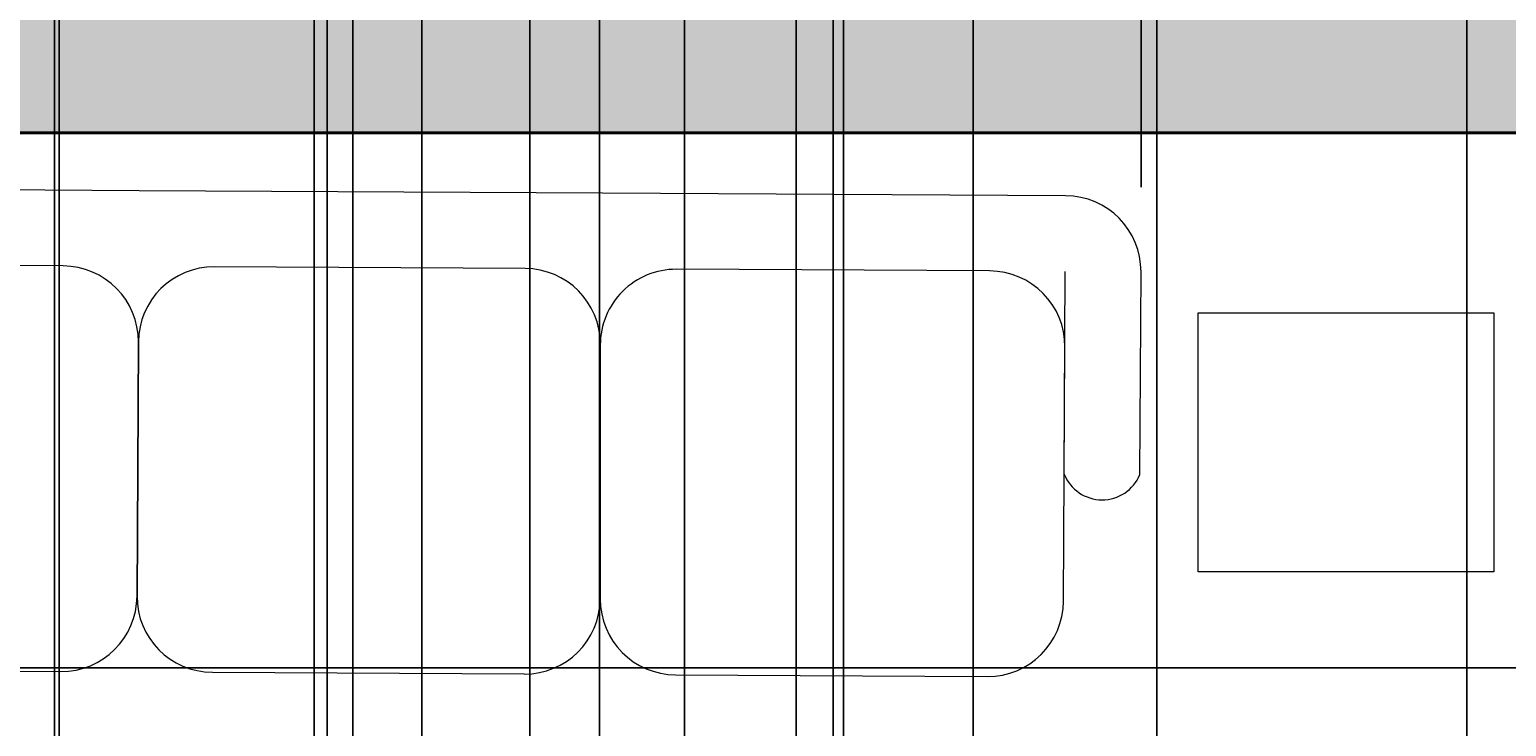
# Model space of a CAD drawing. Units: inches. Extents: x 818 to 1898, y 976 to 2364.
# Tile 31 of 96: x 1282 to 1391, y 1643 to 1695. Entities that reach past the tile are written whole.
import ezdxf

# ---------------------------------------------------------------- set-up
doc = ezdxf.new("R2010")
doc.units = ezdxf.units.IN
doc.header["$LTSCALE"] = 5
doc.header["$MEASUREMENT"] = 0
for name, color, linetype, lineweight in [('A-ANNO-DIMS', 2, 'Continuous', 18), ('A-FURN', 8, 'Continuous', 18), ('A-WALL', 7, 'Continuous', 40)]:
    doc.layers.add(name, color=color, linetype=linetype, lineweight=lineweight)
doc.layers.add('A-WALL-PATT', color=251, linetype='Continuous', lineweight=13, true_color=0x636466)
doc.styles.get("Standard").update_dxf_attribs({"font": 'arial.ttf'})
doc.dimstyles.get("Standard").update_dxf_attribs({"dimtxt": 0.18, "dimasz": 0.18, "dimexe": 0.18, "dimexo": 0.0625, "dimgap": 0.09, "dimtad": 0, "dimtih": 1, "dimtoh": 1, "dimdec": 4, "dimzin": 0, "dimdsep": 46, "dimtxsty": 'Standard', "dimcen": 0.09, "dimadec": 0, "dimazin": 0, "dimtfac": 1, "dimtdec": 4, "dimtofl": 0, "dimtmove": 0, "dimatfit": 3, "dimfxl": 1, "dimtolj": 1, "dimtzin": 0, "dimarcsym": 0})

# ---------------------------------------------------------------- blocks, each defined once
blk = doc.blocks.new('SOFA-3-SEAT')
for p, q in [((39.87, 35.86), (5.7, 36.05)), ((74.05, 35.68), (39.88, 35.86)), ((108.23, 35.49), (74.06, 35.68)), ((34.25, 30.31), (11.25, 30.43)), ((68.34, 30.12), (45.43, 30.24)), ((102.62, 29.94), (79.51, 30.06)), ((108.12, 14.94), (108.2, 29.9)), ((113.71, 14.91), (113.79, 29.87)), ((39.71, 5.93), (39.81, 24.69)), ((39.82, 24.69), (39.72, 5.93)), ((73.9, 5.71), (73.9, 24.47)), ((108.07, 5.56), (108.17, 24.32)), ((11.09, 0.49), (34.09, 0.37)), ((45.27, 0.31), (68.27, 0.19)), ((79.45, 0.12), (102.45, 0))]:
    blk.add_line(p, q)
for centre, radius, start, end in [((108.2, 29.9), 5.59, 359.6898, 89.6898), ((34.22, 24.72), 5.59, 359.6898, 89.6898), ((45.4, 24.66), 5.59, 89.6898, 179.6898), ((68.31, 24.53), 5.59, 0, 89.6898), ((79.48, 24.47), 5.59, 89.6898, 180), ((102.59, 24.35), 5.59, 359.6898, 89.6898), ((110.92, 16.05), 3.01, 201.7034, 337.6762), ((34.12, 5.96), 5.59, 269.6898, 359.6898), ((45.3, 5.9), 5.59, 179.6898, 269.6898), ((68.3, 5.77), 5.59, 269.6898, 359.6898), ((79.48, 5.71), 5.59, 179.6898, 269.6898), ((102.48, 5.59), 5.59, 269.6898, 359.6898)]:
    blk.add_arc(centre, radius, start, end)
blk = doc.blocks.new('SIDE-TABLE')
blk.add_lwpolyline([(0, 19.12), (21.82, 19.12), (21.82, 0), (0, 0)], close=True)
blk = doc.blocks.new('*D42')
at = {"layer": 'A-ANNO-DIMS', "color": 0, "lineweight": -2, "ltscale": 5, "transparency": 16777216}
for p, q in [((1250.19, 1683.07), (1250.19, 1700.26)), ((1250.37, 1700.08), (1306.12, 1700.08)), ((1363.82, 1700.08), (1308.07, 1700.08)), ((1364, 1683.07), (1364, 1700.26))]:
    blk.add_line(p, q, dxfattribs=at)
at = {"layer": 'A-ANNO-DIMS', "color": 0, "ltscale": 5, "transparency": 16777216}
for points in [[(1250.37, 1700.11), (1250.37, 1700.05), (1250.19, 1700.08)], [(1363.82, 1700.11), (1363.82, 1700.05), (1364, 1700.08)]]:
    blk.add_solid(points, dxfattribs=at)
at = {"layer": 'Defpoints', "color": 0, "ltscale": 5, "transparency": 16777216}
for p in [(1364, 1700.08), (1250.19, 1683.01), (1364, 1683.01)]:
    blk.add_point(p, dxfattribs=at)
at = {"layer": 'A-ANNO-DIMS', "color": 0, "ltscale": 5, "transparency": 16777216, "insert": (1307.1, 1700.08), "char_height": 0.18, "attachment_point": 5}
blk.add_mtext('\\A1;SOFA 114 TYP.', dxfattribs=at)
blk = doc.blocks.new('*D61')
at = {"layer": 'A-ANNO-DIMS', "color": 0, "lineweight": -2, "ltscale": 5, "transparency": 16777216}
for p, q in [((1071.73, 1203.03), (1071.73, 2363.87)), ((1071.91, 2363.69), (1250.94, 2363.69)), ((1430.55, 2363.69), (1251.51, 2363.69)), ((1430.73, 1203.03), (1430.73, 2363.87))]:
    blk.add_line(p, q, dxfattribs=at)
at = {"layer": 'A-ANNO-DIMS', "color": 0, "ltscale": 5, "transparency": 16777216}
for points in [[(1071.91, 2363.72), (1071.91, 2363.66), (1071.73, 2363.69)], [(1430.55, 2363.72), (1430.55, 2363.66), (1430.73, 2363.69)]]:
    blk.add_solid(points, dxfattribs=at)
at = {"layer": 'Defpoints', "color": 0, "ltscale": 5, "transparency": 16777216}
for p in [(1430.73, 2363.69), (1071.73, 1202.96), (1430.73, 1202.96)]:
    blk.add_point(p, dxfattribs=at)
at = {"layer": 'A-ANNO-DIMS', "color": 0, "ltscale": 5, "transparency": 16777216, "insert": (1251.23, 2363.69), "char_height": 0.18, "attachment_point": 5}
blk.add_mtext('\\A1;359', dxfattribs=at)
blk = doc.blocks.new('*D64')
at = {"layer": 'A-ANNO-DIMS', "color": 0, "lineweight": -2, "ltscale": 5, "transparency": 16777216}
for p, q in [((1197.73, 1501.14), (1197.73, 2363.87)), ((1197.91, 2363.69), (1313.93, 2363.69)), ((1430.55, 2363.69), (1314.52, 2363.69)), ((1430.73, 1501.14), (1430.73, 2363.87))]:
    blk.add_line(p, q, dxfattribs=at)
at = {"layer": 'A-ANNO-DIMS', "color": 0, "ltscale": 5, "transparency": 16777216}
for points in [[(1197.91, 2363.72), (1197.91, 2363.66), (1197.73, 2363.69)], [(1430.55, 2363.72), (1430.55, 2363.66), (1430.73, 2363.69)]]:
    blk.add_solid(points, dxfattribs=at)
at = {"layer": 'Defpoints', "color": 0, "ltscale": 5, "transparency": 16777216}
for p in [(1430.73, 2363.69), (1197.73, 1501.08), (1430.73, 1501.08)]:
    blk.add_point(p, dxfattribs=at)
at = {"layer": 'A-ANNO-DIMS', "color": 0, "ltscale": 5, "transparency": 16777216, "insert": (1314.23, 2363.69), "char_height": 0.18, "attachment_point": 5}
blk.add_mtext('\\A1;233', dxfattribs=at)
blk = doc.blocks.new('*D96')
at = {"layer": 'A-ANNO-DIMS', "color": 0, "lineweight": -2, "ltscale": 5, "transparency": 16777216}
for p, q in [((1229.65, 1071.12), (1229.65, 2363.87)), ((1229.83, 2363.69), (1256.52, 2363.69)), ((1283.99, 2363.69), (1257.3, 2363.69)), ((1284.17, 1071.12), (1284.17, 2363.87))]:
    blk.add_line(p, q, dxfattribs=at)
at = {"layer": 'A-ANNO-DIMS', "color": 0, "ltscale": 5, "transparency": 16777216}
for points in [[(1229.83, 2363.72), (1229.83, 2363.66), (1229.65, 2363.69)], [(1283.99, 2363.72), (1283.99, 2363.66), (1284.17, 2363.69)]]:
    blk.add_solid(points, dxfattribs=at)
at = {"layer": 'Defpoints', "color": 0, "ltscale": 5, "transparency": 16777216}
for p in [(1284.17, 2363.69), (1229.65, 1071.06), (1284.17, 1071.06)]:
    blk.add_point(p, dxfattribs=at)
at = {"layer": 'A-ANNO-DIMS', "color": 0, "ltscale": 5, "transparency": 16777216, "insert": (1256.91, 2363.69), "char_height": 0.18, "attachment_point": 5}
blk.add_mtext('\\A1;54.52', dxfattribs=at)
blk = doc.blocks.new('*D97')
at = {"layer": 'A-ANNO-DIMS', "color": 0, "lineweight": -2, "ltscale": 5, "transparency": 16777216}
for p, q in [((1284.17, 1071.12), (1284.17, 2363.87)), ((1284.35, 2363.69), (1310.96, 2363.69)), ((1338.36, 2363.69), (1311.75, 2363.69)), ((1338.54, 1071.12), (1338.54, 2363.87))]:
    blk.add_line(p, q, dxfattribs=at)
at = {"layer": 'A-ANNO-DIMS', "color": 0, "ltscale": 5, "transparency": 16777216}
for points in [[(1284.35, 2363.72), (1284.35, 2363.66), (1284.17, 2363.69)], [(1338.36, 2363.72), (1338.36, 2363.66), (1338.54, 2363.69)]]:
    blk.add_solid(points, dxfattribs=at)
at = {"layer": 'Defpoints', "color": 0, "ltscale": 5, "transparency": 16777216}
for p in [(1338.54, 2363.69), (1284.17, 1071.06), (1338.54, 1071.06)]:
    blk.add_point(p, dxfattribs=at)
at = {"layer": 'A-ANNO-DIMS', "color": 0, "ltscale": 5, "transparency": 16777216, "insert": (1311.36, 2363.69), "char_height": 0.18, "attachment_point": 5}
blk.add_mtext('\\A1;54.37', dxfattribs=at)
blk = doc.blocks.new('*D98')
at = {"layer": 'A-ANNO-DIMS', "color": 0, "lineweight": -2, "ltscale": 5, "transparency": 16777216}
for p, q in [((1338.54, 1071.12), (1338.54, 2363.87)), ((1338.72, 2363.69), (1364.81, 2363.69)), ((1391.7, 2363.69), (1365.6, 2363.69)), ((1391.88, 1071.12), (1391.88, 2363.87))]:
    blk.add_line(p, q, dxfattribs=at)
at = {"layer": 'A-ANNO-DIMS', "color": 0, "ltscale": 5, "transparency": 16777216}
for points in [[(1338.72, 2363.72), (1338.72, 2363.66), (1338.54, 2363.69)], [(1391.7, 2363.72), (1391.7, 2363.66), (1391.88, 2363.69)]]:
    blk.add_solid(points, dxfattribs=at)
at = {"layer": 'Defpoints', "color": 0, "ltscale": 5, "transparency": 16777216}
for p in [(1391.88, 2363.69), (1338.54, 1071.06), (1391.88, 1071.06)]:
    blk.add_point(p, dxfattribs=at)
at = {"layer": 'A-ANNO-DIMS', "color": 0, "ltscale": 5, "transparency": 16777216, "insert": (1365.21, 2363.69), "char_height": 0.18, "attachment_point": 5}
blk.add_mtext('\\A1;53.33', dxfattribs=at)
blk = doc.blocks.new('*D119')
at = {"layer": 'A-ANNO-DIMS', "color": 0, "lineweight": -2, "ltscale": 5, "transparency": 16777216}
for p, q in [((1766.29, 1716.99), (818.03, 1716.99)), ((818.21, 1716.81), (818.21, 1672.43)), ((818.21, 1627.69), (818.21, 1672.06)), ((1766.29, 1627.51), (818.03, 1627.51))]:
    blk.add_line(p, q, dxfattribs=at)
at = {"layer": 'A-ANNO-DIMS', "color": 0, "ltscale": 5, "transparency": 16777216}
for points in [[(818.18, 1716.81), (818.24, 1716.81), (818.21, 1716.99)], [(818.18, 1627.69), (818.24, 1627.69), (818.21, 1627.51)]]:
    blk.add_solid(points, dxfattribs=at)
at = {"layer": 'Defpoints', "color": 0, "ltscale": 5, "transparency": 16777216}
for p in [(818.21, 1716.99), (1766.35, 1716.99), (1766.35, 1627.51)]:
    blk.add_point(p, dxfattribs=at)
at = {"layer": 'A-ANNO-DIMS', "color": 0, "ltscale": 5, "transparency": 16777216, "insert": (818.21, 1672.25), "char_height": 0.18, "attachment_point": 5}
blk.add_mtext('\\A1;89.48', dxfattribs=at)
blk = doc.blocks.new('*D159')
at = {"layer": 'A-ANNO-DIMS', "color": 0, "lineweight": -2, "ltscale": 5, "transparency": 16777216}
for p, q in [((1206.73, 1687.02), (1206.73, 975.66)), ((1463.73, 1687.02), (1463.73, 975.66)), ((1206.91, 975.84), (1334.93, 975.84)), ((1463.55, 975.84), (1335.52, 975.84))]:
    blk.add_line(p, q, dxfattribs=at)
at = {"layer": 'A-ANNO-DIMS', "color": 0, "ltscale": 5, "transparency": 16777216}
for points in [[(1206.91, 975.87), (1206.91, 975.81), (1206.73, 975.84)], [(1463.55, 975.87), (1463.55, 975.81), (1463.73, 975.84)]]:
    blk.add_solid(points, dxfattribs=at)
at = {"layer": 'Defpoints', "color": 0, "ltscale": 5, "transparency": 16777216}
for p in [(1206.73, 1687.08), (1463.73, 1687.08), (1463.73, 975.84)]:
    blk.add_point(p, dxfattribs=at)
at = {"layer": 'A-ANNO-DIMS', "color": 0, "ltscale": 5, "transparency": 16777216, "insert": (1335.23, 975.84), "char_height": 0.18, "attachment_point": 5}
blk.add_mtext('\\A1;257', dxfattribs=at)
blk = doc.blocks.new('*D165')
at = {"layer": 'A-ANNO-DIMS', "color": 0, "lineweight": -2, "ltscale": 5, "transparency": 16777216}
for p, q in [((1283.82, 1510.14), (1283.82, 2363.87)), ((1284, 2363.69), (1324.09, 2363.69)), ((1364.97, 2363.69), (1324.88, 2363.69)), ((1365.15, 1510.14), (1365.15, 2363.87))]:
    blk.add_line(p, q, dxfattribs=at)
at = {"layer": 'A-ANNO-DIMS', "color": 0, "ltscale": 5, "transparency": 16777216}
for points in [[(1284, 2363.72), (1284, 2363.66), (1283.82, 2363.69)], [(1364.97, 2363.72), (1364.97, 2363.66), (1365.15, 2363.69)]]:
    blk.add_solid(points, dxfattribs=at)
at = {"layer": 'Defpoints', "color": 0, "ltscale": 5, "transparency": 16777216}
for p in [(1365.15, 2363.69), (1283.82, 1510.08), (1365.15, 1510.08)]:
    blk.add_point(p, dxfattribs=at)
at = {"layer": 'A-ANNO-DIMS', "color": 0, "ltscale": 5, "transparency": 16777216, "insert": (1324.48, 2363.69), "char_height": 0.18, "attachment_point": 5}
blk.add_mtext('\\A1;81.33', dxfattribs=at)
blk = doc.blocks.new('*D176')
at = {"layer": 'A-ANNO-DIMS', "color": 0, "lineweight": -2, "ltscale": 5, "transparency": 16777216}
for p, q in [((1559.66, 1687.08), (818.03, 1687.08)), ((818.21, 1686.9), (818.21, 1667.51)), ((818.21, 1647.76), (818.21, 1667.15)), ((1559.66, 1647.58), (818.03, 1647.58))]:
    blk.add_line(p, q, dxfattribs=at)
at = {"layer": 'A-ANNO-DIMS', "color": 0, "ltscale": 5, "transparency": 16777216}
for points in [[(818.18, 1686.9), (818.24, 1686.9), (818.21, 1687.08)], [(818.18, 1647.76), (818.24, 1647.76), (818.21, 1647.58)]]:
    blk.add_solid(points, dxfattribs=at)
at = {"layer": 'Defpoints', "color": 0, "ltscale": 5, "transparency": 16777216}
for p in [(1559.73, 1687.08), (818.21, 1647.58), (1559.73, 1647.58)]:
    blk.add_point(p, dxfattribs=at)
at = {"layer": 'A-ANNO-DIMS', "color": 0, "ltscale": 5, "transparency": 16777216, "insert": (818.21, 1667.33), "char_height": 0.18, "attachment_point": 5}
blk.add_mtext('\\A1;39.5', dxfattribs=at)
blk = doc.blocks.new('*D215')
at = {"layer": 'A-ANNO-DIMS', "color": 0, "lineweight": -2, "ltscale": 5, "transparency": 16777216}
for p, q in [((1590.66, 1876.08), (818.03, 1876.08)), ((818.21, 1875.9), (818.21, 1781.76)), ((818.21, 1687.26), (818.21, 1781.4)), ((1511.66, 1687.08), (818.03, 1687.08))]:
    blk.add_line(p, q, dxfattribs=at)
at = {"layer": 'A-ANNO-DIMS', "color": 0, "ltscale": 5, "transparency": 16777216}
for points in [[(818.18, 1875.9), (818.24, 1875.9), (818.21, 1876.08)], [(818.18, 1687.26), (818.24, 1687.26), (818.21, 1687.08)]]:
    blk.add_solid(points, dxfattribs=at)
at = {"layer": 'Defpoints', "color": 0, "ltscale": 5, "transparency": 16777216}
for p in [(818.21, 1876.08), (1590.73, 1876.08), (1511.73, 1687.08)]:
    blk.add_point(p, dxfattribs=at)
at = {"layer": 'A-ANNO-DIMS', "color": 0, "ltscale": 5, "transparency": 16777216, "insert": (818.21, 1781.58), "char_height": 0.18, "attachment_point": 5}
blk.add_mtext('\\A1;189', dxfattribs=at)
blk = doc.blocks.new('*D231')
at = {"layer": 'A-ANNO-DIMS', "color": 0, "lineweight": -2, "ltscale": 5, "transparency": 16777216}
for p, q in [((1303.93, 1952.98), (1303.93, 975.66)), ((1402.52, 1952.98), (1402.52, 975.66)), ((1304.11, 975.84), (1352.83, 975.84)), ((1402.34, 975.84), (1353.62, 975.84))]:
    blk.add_line(p, q, dxfattribs=at)
at = {"layer": 'A-ANNO-DIMS', "color": 0, "ltscale": 5, "transparency": 16777216}
for points in [[(1304.11, 975.87), (1304.11, 975.81), (1303.93, 975.84)], [(1402.34, 975.87), (1402.34, 975.81), (1402.52, 975.84)]]:
    blk.add_solid(points, dxfattribs=at)
at = {"layer": 'Defpoints', "color": 0, "ltscale": 5, "transparency": 16777216}
for p in [(1303.93, 1953.04), (1402.52, 1953.04), (1402.52, 975.84)]:
    blk.add_point(p, dxfattribs=at)
at = {"layer": 'A-ANNO-DIMS', "color": 0, "ltscale": 5, "transparency": 16777216, "insert": (1353.22, 975.84), "char_height": 0.18, "attachment_point": 5}
blk.add_mtext('\\A1;98.59', dxfattribs=at)
blk = doc.blocks.new('*D233')
at = {"layer": 'A-ANNO-DIMS', "color": 0, "lineweight": -2, "ltscale": 5, "transparency": 16777216}
for p, q in [((1267.73, 2044.02), (1267.73, 975.66)), ((1303.93, 2008.33), (1303.93, 975.66)), ((1267.91, 975.84), (1285.36, 975.84)), ((1303.75, 975.84), (1286.29, 975.84))]:
    blk.add_line(p, q, dxfattribs=at)
at = {"layer": 'A-ANNO-DIMS', "color": 0, "ltscale": 5, "transparency": 16777216}
for points in [[(1267.91, 975.87), (1267.91, 975.81), (1267.73, 975.84)], [(1303.75, 975.87), (1303.75, 975.81), (1303.93, 975.84)]]:
    blk.add_solid(points, dxfattribs=at)
at = {"layer": 'Defpoints', "color": 0, "ltscale": 5, "transparency": 16777216}
for p in [(1267.73, 2044.08), (1303.93, 2008.39), (1303.93, 975.84)]:
    blk.add_point(p, dxfattribs=at)
at = {"layer": 'A-ANNO-DIMS', "color": 0, "ltscale": 5, "transparency": 16777216, "insert": (1285.83, 975.84), "char_height": 0.18, "attachment_point": 5}
blk.add_mtext('\\A1;36.206', dxfattribs=at)
blk = doc.blocks.new('*D236')
at = {"layer": 'A-ANNO-DIMS', "color": 0, "lineweight": -2, "ltscale": 5, "transparency": 16777216}
for p, q in [((1310.91, 2026.14), (1310.91, 975.66)), ((1342.04, 2026.14), (1342.04, 975.66)), ((1311.09, 975.84), (1326.08, 975.84)), ((1341.86, 975.84), (1326.87, 975.84))]:
    blk.add_line(p, q, dxfattribs=at)
at = {"layer": 'A-ANNO-DIMS', "color": 0, "ltscale": 5, "transparency": 16777216}
for points in [[(1311.09, 975.87), (1311.09, 975.81), (1310.91, 975.84)], [(1341.86, 975.87), (1341.86, 975.81), (1342.04, 975.84)]]:
    blk.add_solid(points, dxfattribs=at)
at = {"layer": 'Defpoints', "color": 0, "ltscale": 5, "transparency": 16777216}
for p in [(1310.91, 2026.21), (1342.04, 2026.21), (1342.04, 975.84)]:
    blk.add_point(p, dxfattribs=at)
at = {"layer": 'A-ANNO-DIMS', "color": 0, "ltscale": 5, "transparency": 16777216, "insert": (1326.48, 975.84), "char_height": 0.18, "attachment_point": 5}
blk.add_mtext('\\A1;31.14', dxfattribs=at)
blk = doc.blocks.new('*D252')
at = {"layer": 'A-ANNO-DIMS', "color": 0, "lineweight": -2, "ltscale": 5, "transparency": 16777216}
for p, q in [((1330.3, 2053.02), (1330.3, 975.66)), ((1388.03, 2053.02), (1388.03, 975.66)), ((1330.48, 975.84), (1358.77, 975.84)), ((1387.85, 975.84), (1359.56, 975.84))]:
    blk.add_line(p, q, dxfattribs=at)
at = {"layer": 'A-ANNO-DIMS', "color": 0, "ltscale": 5, "transparency": 16777216}
for points in [[(1330.48, 975.87), (1330.48, 975.81), (1330.3, 975.84)], [(1387.85, 975.87), (1387.85, 975.81), (1388.03, 975.84)]]:
    blk.add_solid(points, dxfattribs=at)
at = {"layer": 'Defpoints', "color": 0, "ltscale": 5, "transparency": 16777216}
for p in [(1330.3, 2053.08), (1388.03, 2053.08), (1388.03, 975.84)]:
    blk.add_point(p, dxfattribs=at)
at = {"layer": 'A-ANNO-DIMS', "color": 0, "ltscale": 5, "transparency": 16777216, "insert": (1359.17, 975.84), "char_height": 0.18, "attachment_point": 5}
blk.add_mtext('\\A1;57.73', dxfattribs=at)
blk = doc.blocks.new('*D254')
at = {"layer": 'A-ANNO-DIMS', "color": 0, "lineweight": -2, "ltscale": 5, "transparency": 16777216}
for p, q in [((1267.73, 2044.02), (1267.73, 975.66)), ((1330.3, 2044.02), (1330.3, 975.66)), ((1267.91, 975.84), (1298.62, 975.84)), ((1330.12, 975.84), (1299.41, 975.84))]:
    blk.add_line(p, q, dxfattribs=at)
at = {"layer": 'A-ANNO-DIMS', "color": 0, "ltscale": 5, "transparency": 16777216}
for points in [[(1267.91, 975.87), (1267.91, 975.81), (1267.73, 975.84)], [(1330.12, 975.87), (1330.12, 975.81), (1330.3, 975.84)]]:
    blk.add_solid(points, dxfattribs=at)
at = {"layer": 'Defpoints', "color": 0, "ltscale": 5, "transparency": 16777216}
for p in [(1267.73, 2044.08), (1330.3, 2044.08), (1330.3, 975.84)]:
    blk.add_point(p, dxfattribs=at)
at = {"layer": 'A-ANNO-DIMS', "color": 0, "ltscale": 5, "transparency": 16777216, "insert": (1299.02, 975.84), "char_height": 0.18, "attachment_point": 5}
blk.add_mtext('\\A1;62.58', dxfattribs=at)
blk = doc.blocks.new('*D269')
at = {"layer": 'A-ANNO-DIMS', "color": 0, "lineweight": -2, "ltscale": 5, "transparency": 16777216}
for p, q in [((1246.94, 1534.14), (1246.94, 2363.87)), ((1247.12, 2363.69), (1293.71, 2363.69)), ((1341.08, 2363.69), (1294.49, 2363.69)), ((1341.26, 1534.14), (1341.26, 2363.87))]:
    blk.add_line(p, q, dxfattribs=at)
at = {"layer": 'A-ANNO-DIMS', "color": 0, "ltscale": 5, "transparency": 16777216}
for points in [[(1247.12, 2363.72), (1247.12, 2363.66), (1246.94, 2363.69)], [(1341.08, 2363.72), (1341.08, 2363.66), (1341.26, 2363.69)]]:
    blk.add_solid(points, dxfattribs=at)
at = {"layer": 'Defpoints', "color": 0, "ltscale": 5, "transparency": 16777216}
for p in [(1341.26, 2363.69), (1246.94, 1534.08), (1341.26, 1534.08)]:
    blk.add_point(p, dxfattribs=at)
at = {"layer": 'A-ANNO-DIMS', "color": 0, "ltscale": 5, "transparency": 16777216, "insert": (1294.1, 2363.69), "char_height": 0.18, "attachment_point": 5}
blk.add_mtext('\\A1;94.32', dxfattribs=at)
blk = doc.blocks.new('*D278')
at = {"layer": 'A-ANNO-DIMS', "color": 0, "lineweight": -2, "ltscale": 5, "transparency": 16777216}
for p, q in [((1324.03, 1700.74), (1324.03, 975.66)), ((1267.73, 1696.02), (1267.73, 975.66)), ((1267.91, 975.84), (1295.5, 975.84)), ((1323.85, 975.84), (1296.26, 975.84))]:
    blk.add_line(p, q, dxfattribs=at)
at = {"layer": 'A-ANNO-DIMS', "color": 0, "ltscale": 5, "transparency": 16777216}
for points in [[(1267.91, 975.87), (1267.91, 975.81), (1267.73, 975.84)], [(1323.85, 975.87), (1323.85, 975.81), (1324.03, 975.84)]]:
    blk.add_solid(points, dxfattribs=at)
at = {"layer": 'Defpoints', "color": 0, "ltscale": 5, "transparency": 16777216}
for p in [(1324.03, 1700.81), (1267.73, 1696.08), (1324.03, 975.84)]:
    blk.add_point(p, dxfattribs=at)
at = {"layer": 'A-ANNO-DIMS', "color": 0, "ltscale": 5, "transparency": 16777216, "insert": (1295.88, 975.84), "char_height": 0.18, "attachment_point": 5}
blk.add_mtext('\\A1;56.31', dxfattribs=at)
blk = doc.blocks.new('*D283')
at = {"layer": 'A-ANNO-DIMS', "color": 0, "lineweight": -2, "ltscale": 5, "transparency": 16777216}
for p, q in [((1351.6, 1761.39), (1351.6, 975.66)), ((1267.73, 1696.02), (1267.73, 975.66)), ((1267.91, 975.84), (1309.27, 975.84)), ((1351.42, 975.84), (1310.06, 975.84))]:
    blk.add_line(p, q, dxfattribs=at)
at = {"layer": 'A-ANNO-DIMS', "color": 0, "ltscale": 5, "transparency": 16777216}
for points in [[(1267.91, 975.87), (1267.91, 975.81), (1267.73, 975.84)], [(1351.42, 975.87), (1351.42, 975.81), (1351.6, 975.84)]]:
    blk.add_solid(points, dxfattribs=at)
at = {"layer": 'Defpoints', "color": 0, "ltscale": 5, "transparency": 16777216}
for p in [(1351.6, 1761.45), (1267.73, 1696.08), (1351.6, 975.84)]:
    blk.add_point(p, dxfattribs=at)
at = {"layer": 'A-ANNO-DIMS', "color": 0, "ltscale": 5, "transparency": 16777216, "insert": (1309.66, 975.84), "char_height": 0.18, "attachment_point": 5}
blk.add_mtext('\\A1;83.87', dxfattribs=at)
blk = doc.blocks.new('*D285')
at = {"layer": 'A-ANNO-DIMS', "color": 0, "lineweight": -2, "ltscale": 5, "transparency": 16777216}
for p, q in [((1305.83, 1830.02), (1305.83, 975.66)), ((1267.73, 1814.9), (1267.73, 975.66)), ((1267.91, 975.84), (1286.47, 975.84)), ((1305.65, 975.84), (1287.08, 975.84))]:
    blk.add_line(p, q, dxfattribs=at)
at = {"layer": 'A-ANNO-DIMS', "color": 0, "ltscale": 5, "transparency": 16777216}
for points in [[(1267.91, 975.87), (1267.91, 975.81), (1267.73, 975.84)], [(1305.65, 975.87), (1305.65, 975.81), (1305.83, 975.84)]]:
    blk.add_solid(points, dxfattribs=at)
at = {"layer": 'Defpoints', "color": 0, "ltscale": 5, "transparency": 16777216}
for p in [(1305.83, 1830.08), (1267.73, 1814.97), (1267.73, 975.84)]:
    blk.add_point(p, dxfattribs=at)
at = {"layer": 'A-ANNO-DIMS', "color": 0, "ltscale": 5, "transparency": 16777216, "insert": (1286.78, 975.84), "char_height": 0.18, "attachment_point": 5}
blk.add_mtext('\\A1;38.1', dxfattribs=at)
blk = doc.blocks.new('*D290')
at = {"layer": 'A-ANNO-DIMS', "color": 0, "lineweight": -2, "ltscale": 5, "transparency": 16777216}
for p, q in [((1302.98, 1599.43), (1302.98, 2363.87)), ((1303.16, 2363.69), (1310.57, 2363.69)), ((1318.71, 2363.69), (1311.31, 2363.69)), ((1318.89, 1607.83), (1318.89, 2363.87))]:
    blk.add_line(p, q, dxfattribs=at)
at = {"layer": 'A-ANNO-DIMS', "color": 0, "ltscale": 5, "transparency": 16777216}
for points in [[(1303.16, 2363.72), (1303.16, 2363.66), (1302.98, 2363.69)], [(1318.71, 2363.72), (1318.71, 2363.66), (1318.89, 2363.69)]]:
    blk.add_solid(points, dxfattribs=at)
at = {"layer": 'Defpoints', "color": 0, "ltscale": 5, "transparency": 16777216}
for p in [(1318.89, 2363.69), (1318.89, 1607.77), (1302.98, 1599.37)]:
    blk.add_point(p, dxfattribs=at)
at = {"layer": 'A-ANNO-DIMS', "color": 0, "ltscale": 5, "transparency": 16777216, "insert": (1310.94, 2363.69), "char_height": 0.18, "attachment_point": 5}
blk.add_mtext('\\A1;15.91', dxfattribs=at)
blk = doc.blocks.new('*D291')
at = {"layer": 'A-ANNO-DIMS', "color": 0, "lineweight": -2, "ltscale": 5, "transparency": 16777216}
for p, q in [((1206.79, 1687.08), (1897.92, 1687.08)), ((1897.74, 1686.9), (1897.74, 1647.61)), ((1897.74, 1607.95), (1897.74, 1647.24)), ((1318.96, 1607.77), (1897.92, 1607.77))]:
    blk.add_line(p, q, dxfattribs=at)
at = {"layer": 'A-ANNO-DIMS', "color": 0, "ltscale": 5, "transparency": 16777216}
for points in [[(1897.71, 1686.9), (1897.77, 1686.9), (1897.74, 1687.08)], [(1897.71, 1607.95), (1897.77, 1607.95), (1897.74, 1607.77)]]:
    blk.add_solid(points, dxfattribs=at)
at = {"layer": 'Defpoints', "color": 0, "ltscale": 5, "transparency": 16777216}
for p in [(1206.73, 1687.08), (1897.74, 1687.08), (1318.89, 1607.77)]:
    blk.add_point(p, dxfattribs=at)
at = {"layer": 'A-ANNO-DIMS', "color": 0, "ltscale": 5, "transparency": 16777216, "insert": (1897.74, 1647.42), "char_height": 0.18, "attachment_point": 5}
blk.add_mtext('\\A1;79.3', dxfattribs=at)

msp = doc.modelspace()

# ---------------------------------------------------------------- hatches: boundary and pattern name
at = {"layer": 'A-WALL-PATT', "ltscale": 5}
h = msp.add_hatch(color=256, dxfattribs=at)
h.dxf.hatch_style = 1
h.paths.add_polyline_path([(1267.7251, 1928.9218), (1258.7252, 1928.9218), (1258.7252, 1913.6401), (1250.3029, 1913.6401), (1250.3029, 1878.3919), (1258.7252, 1878.3919), (1258.7252, 1862.9652), (1267.7251, 1862.9652)])
h.paths.add_polyline_path([(1267.7251, 1814.9652), (1258.7252, 1814.9652), (1258.7252, 1755.3321), (1267.7251, 1755.3321)])
h.paths.add_polyline_path([(1463.7251, 1696.0782), (1267.7251, 1696.0782), (1267.7251, 1707.3321), (1258.7252, 1707.3321), (1258.7252, 1700.0782), (1251.9333, 1700.0782), (1251.9333, 1687.0782), (1463.7251, 1687.0782)])
h.paths.add_polyline_path([(1714.7252, 1717.3178), (1705.7252, 1717.3178), (1705.7252, 1696.0782), (1599.7252, 1696.0782), (1599.7252, 1790.0782), (1705.7252, 1790.0782), (1705.7252, 1785.6125), (1714.7252, 1785.6125), (1714.7252, 1827.2125), (1705.7252, 1827.2125), (1705.7252, 1802.0782), (1599.7252, 1802.0782), (1599.7252, 1867.0782), (1705.7252, 1867.0782), (1705.7252, 1857.2125), (1714.7252, 1857.2125), (1714.7252, 1930.0316), (1741.8409, 1930.0316), (1741.8409, 1935.0316), (1714.7252, 1935.0316), (1714.7252, 1957.0338), (1741.8409, 1957.0338), (1741.8409, 1962.0338), (1714.7252, 1962.0338), (1705.7252, 1962.0338), (1705.7252, 1948.0782), (1599.7252, 1948.0782), (1599.7252, 1981.0782), (1590.7251, 1981.0782), (1590.7251, 1941.0782), (1620.7252, 1941.0782), (1705.7252, 1941.0782), (1705.7252, 1876.0782), (1599.7252, 1876.0782), (1599.7252, 1911.0782), (1590.7251, 1911.0782), (1590.7251, 1876.0782), (1429.2252, 1876.0782), (1429.2252, 1867.0782), (1511.7251, 1867.0782), (1528.593, 1867.0782), (1595.7252, 1867.0782), (1595.7252, 1773.0782), (1520.7252, 1773.0782), (1520.7252, 1837.5823), (1532.593, 1837.5823), (1532.593, 1867.0782), (1528.593, 1867.0782), (1528.593, 1841.5823), (1511.7251, 1841.5823), (1511.7251, 1744.9714), (1520.7252, 1744.9714), (1520.7252, 1761.0782), (1595.7252, 1761.0782), (1595.7252, 1696.0782), (1520.7252, 1696.0782), (1520.7252, 1716.0454), (1511.7251, 1716.0454), (1511.7251, 1696.0782), (1511.7251, 1687.0782), (1714.7252, 1687.0782)])
h.paths.add_polyline_path([(1714.7252, 2053.0782), (1714.7252, 2081.1881), (1709.7252, 2081.1881), (1709.7252, 2053.0782), (1681.6446, 2053.0782), (1681.6446, 2081.1881), (1676.6446, 2081.1881), (1676.6446, 2053.0782), (1538.5155, 2053.0782), (1538.5155, 2044.0782), (1590.7251, 2044.0782), (1590.7251, 2011.0782), (1599.7252, 2011.0782), (1599.7252, 2044.0782), (1705.7252, 2044.0782), (1705.7252, 2014.5114), (1714.7252, 2014.5114)])
h.paths.add_polyline_path([(1485.1216, 2053.0782), (1422.02, 2053.0782), (1422.02, 2081.1881), (1413.02, 2081.1881), (1413.02, 2053.0782), (1399.6356, 2053.0782), (1399.6356, 2081.1881), (1390.6356, 2081.1881), (1390.6356, 2053.0782), (1388.0315, 2053.0782), (1388.0315, 2044.0782), (1416.2743, 2044.0782), (1485.1216, 2044.0782)])
h.paths.add_polyline_path([(1330.305, 2053.0782), (1258.7252, 2053.0782), (1258.7252, 2019.2871), (1267.7251, 2019.2871), (1267.7251, 2044.0782), (1330.305, 2044.0782)])
h.paths.add_polyline_path([(1258.7252, 2053.0782), (1214.6577, 2053.0782), (1214.6577, 2044.0782), (1258.7252, 2044.0782)])
h.paths.add_polyline_path([(1214.6577, 2053.0782), (1180.349, 2053.0782), (1180.349, 2044.0782), (1214.6577, 2044.0782)])
h.paths.add_polyline_path([(1714.7252, 1639.5782), (1741.8409, 1639.5782), (1741.8409, 1643.5782), (1714.7252, 1643.5782), (1714.7252, 1649.9029), (1705.7252, 1649.9029), (1705.7252, 1600.0782), (1477.7252, 1600.0782), (1477.7252, 1591.0782), (1520.7252, 1591.0782), (1616.7252, 1591.0782), (1616.7252, 1416.6857), (1622.7252, 1416.6857), (1622.7252, 1463.0782), (1624.7252, 1463.0782), (1624.7252, 1467.0782), (1622.7252, 1467.0782), (1622.7252, 1591.0782), (1705.7252, 1591.0782), (1705.7252, 1545.0782), (1714.7252, 1545.0782), (1741.8409, 1545.0782), (1741.8409, 1549.0782), (1714.7252, 1549.0782), (1714.7252, 1593.9175), (1737.8409, 1593.9175), (1737.8409, 1597.9175), (1714.7252, 1597.9175)])
h.paths.add_polyline_path([(1674.9024, 2060.7419), (1714.7045, 2060.7419), (1714.7045, 2073.1061), (1674.9024, 2073.1061)], flags=25)
h.paths.add_polyline_path([(1394.5468, 2061.6618), (1422.2344, 2061.6618), (1422.2344, 2074.0261), (1394.5468, 2074.0261)], flags=24)

# ---------------------------------------------------------------- linework, layer by layer
at = {"layer": 'A-WALL'}
msp.add_line((1206.7251, 1687.0782), (1463.7251, 1687.0782), dxfattribs=at)

# ---------------------------------------------------------------- block references
at = {"layer": 'A-FURN'}
for name, p in [('SOFA-3-SEAT', (1250.195, 1646.945)), ('SIDE-TABLE', (1368.2007, 1654.674))]:
    msp.add_blockref(name, p, dxfattribs=at)

# ---------------------------------------------------------------- dimensions: what is measured, and where the dimension line sits
at = {"layer": 'A-ANNO-DIMS', "ltscale": 5}
for base, p1, p2, override, picture, middle in [((1430.7251, 2363.6929), (1071.7251, 1202.9642), (1430.7251, 1202.9642), {"dimdec": 0, "dimlfac": 1, "dimrnd": 0, "dimzin": 0, "dimdsep": 46, "dimlunit": 2}, '*D61', (1251.2251, 2363.6929)), ((1430.7251, 2363.6929), (1197.7251, 1501.0782), (1430.7251, 1501.0782), {"dimdec": 0, "dimlfac": 1, "dimrnd": 0, "dimzin": 0, "dimdsep": 46, "dimlunit": 2}, '*D64', (1314.2251, 2363.6929)), ((1284.1697, 2363.6929), (1229.6474, 1071.0552), (1284.1697, 1071.0552), {"dimdec": 2, "dimlfac": 1, "dimrnd": 0, "dimzin": 0, "dimdsep": 46, "dimlunit": 2}, '*D96', (1256.9085, 2363.6929)), ((1341.2593, 2363.6929), (1246.9377, 1534.0782), (1341.2593, 1534.0782), {"dimdec": 2, "dimlfac": 1, "dimrnd": 0, "dimzin": 0, "dimdsep": 46, "dimlunit": 2}, '*D269', (1294.0985, 2363.6929)), ((1365.1463, 2363.6929), (1283.8183, 1510.0782), (1365.1463, 1510.0782), {"dimdec": 2, "dimlfac": 1, "dimrnd": 0, "dimzin": 0, "dimdsep": 46, "dimlunit": 2}, '*D165', (1324.4823, 2363.6929)), ((1338.5412, 2363.6929), (1284.1697, 1071.0552), (1338.5412, 1071.0552), {"dimdec": 2, "dimlfac": 1, "dimrnd": 0, "dimzin": 0, "dimdsep": 46, "dimlunit": 2}, '*D97', (1311.3554, 2363.6929)), ((1318.8931, 2363.6929), (1302.9835, 1599.3725), (1318.8931, 1607.7707), {"dimdec": 2, "dimlfac": 1, "dimrnd": 0, "dimzin": 0, "dimdsep": 46, "dimlunit": 2}, '*D290', (1310.9383, 2363.6929)), ((1391.8757, 2363.6929), (1338.5412, 1071.0552), (1391.8757, 1071.0552), {"dimdec": 2, "dimlfac": 1, "dimrnd": 0, "dimzin": 0, "dimdsep": 46, "dimlunit": 2}, '*D98', (1365.2084, 2363.6929)), ((1388.0315, 975.8433), (1330.305, 2053.0782), (1388.0315, 2053.0782), {"dimdec": 2, "dimlfac": 1, "dimrnd": 0, "dimzin": 0, "dimdsep": 46, "dimlunit": 2}, '*D252', (1359.1682, 975.8433)), ((1303.9314, 975.8433), (1267.7251, 2044.0782), (1303.9314, 2008.3917), {"dimdec": 3, "dimlfac": 1, "dimrnd": 0, "dimzin": 0, "dimdsep": 46, "dimlunit": 2}, '*D233', (1285.8283, 975.8433)), ((1330.305, 975.8433), (1267.7251, 2044.0782), (1330.305, 2044.0782), {"dimdec": 2, "dimlfac": 1, "dimrnd": 0, "dimzin": 0, "dimdsep": 46, "dimlunit": 2}, '*D254', (1299.0151, 975.8433)), ((1342.0448, 975.8433), (1310.9077, 2026.2074), (1342.0448, 2026.2074), {"dimdec": 2, "dimlfac": 1, "dimrnd": 0, "dimzin": 0, "dimdsep": 46, "dimlunit": 2}, '*D236', (1326.4762, 975.8433)), ((1402.518, 975.8433), (1303.9314, 1953.0408), (1402.518, 1953.0408), {"dimdec": 2, "dimlfac": 1, "dimrnd": 0, "dimzin": 0, "dimdsep": 46, "dimlunit": 2}, '*D231', (1353.2247, 975.8433)), ((1267.7251, 975.8433), (1305.8278, 1830.0844), (1267.7251, 1814.9652), {"dimdec": 1, "dimlfac": 1, "dimrnd": 0, "dimzin": 0, "dimdsep": 46, "dimlunit": 2}, '*D285', (1286.7765, 975.8433)), ((1351.5985, 975.8433), (1267.7251, 1696.0782), (1351.5985, 1761.449), {"dimdec": 2, "dimlfac": 1, "dimrnd": 0, "dimzin": 0, "dimdsep": 46, "dimlunit": 2}, '*D283', (1309.6618, 975.8433)), ((1324.0334, 975.8433), (1267.7251, 1696.0782), (1324.0334, 1700.8059), {"dimdec": 2, "dimlfac": 1, "dimrnd": 0, "dimzin": 0, "dimdsep": 46, "dimlunit": 2}, '*D278', (1295.8793, 975.8433)), ((1463.7251, 975.8433), (1206.7251, 1687.0782), (1463.7251, 1687.0782), {"dimdec": 0, "dimlfac": 1, "dimrnd": 0, "dimzin": 0, "dimdsep": 46, "dimlunit": 2}, '*D159', (1335.2251, 975.8433))]:
    dim = msp.add_linear_dim(base=base, p1=p1, p2=p2, dimstyle='Standard', override=override, dxfattribs=at)
    dim.commit()
    dim.dimension.update_dxf_attribs({"geometry": picture, "text_midpoint": middle})
for base, p1, p2, override, picture, middle in [((818.2059, 1876.0782), (1511.7251, 1687.0782), (1590.7251, 1876.0782), {"dimdec": 0, "dimlfac": 1, "dimrnd": 0, "dimzin": 0, "dimdsep": 46, "dimlunit": 2}, '*D215', (818.2059, 1781.5782)), ((818.2059, 1716.9866), (1766.3524, 1627.5052), (1766.3524, 1716.9866), {"dimdec": 2, "dimlfac": 1, "dimrnd": 0, "dimzin": 0, "dimdsep": 46, "dimlunit": 2}, '*D119', (818.2059, 1672.2459)), ((818.2059, 1647.5782), (1559.7251, 1687.0782), (1559.7251, 1647.5782), {"dimdec": 1, "dimlfac": 1, "dimrnd": 0, "dimzin": 0, "dimdsep": 46, "dimlunit": 2}, '*D176', (818.2059, 1667.3282)), ((1897.736, 1687.0782), (1318.8931, 1607.7707), (1206.7251, 1687.0782), {"dimdec": 1, "dimlfac": 1, "dimrnd": 0, "dimzin": 0, "dimdsep": 46, "dimlunit": 2}, '*D291', (1897.736, 1647.4245))]:
    dim = msp.add_linear_dim(base=base, p1=p1, p2=p2, angle=90, dimstyle='Standard', override=override, dxfattribs=at)
    dim.commit()
    dim.dimension.update_dxf_attribs({"geometry": picture, "text_midpoint": middle})
dim = msp.add_linear_dim(base=(1364, 1700.0786), p1=(1250.1947, 1683.0078), p2=(1364, 1683.0078), text='SOFA <> TYP.', dimstyle='Standard', override={"dimdec": 0, "dimlfac": 1, "dimrnd": 0, "dimzin": 0, "dimdsep": 46, "dimlunit": 2}, dxfattribs=at)
dim.commit()
dim.dimension.update_dxf_attribs({"geometry": '*D42', "text_midpoint": (1307.0974, 1700.0786)})

doc.saveas('drawing.dxf')
